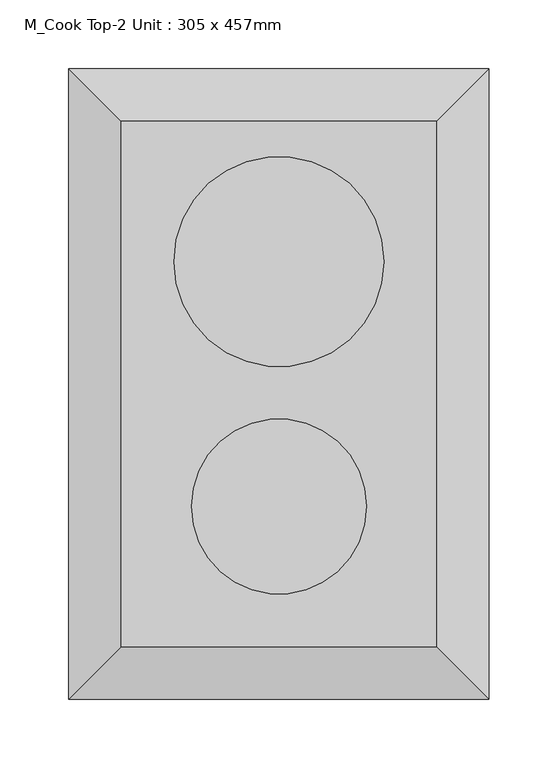
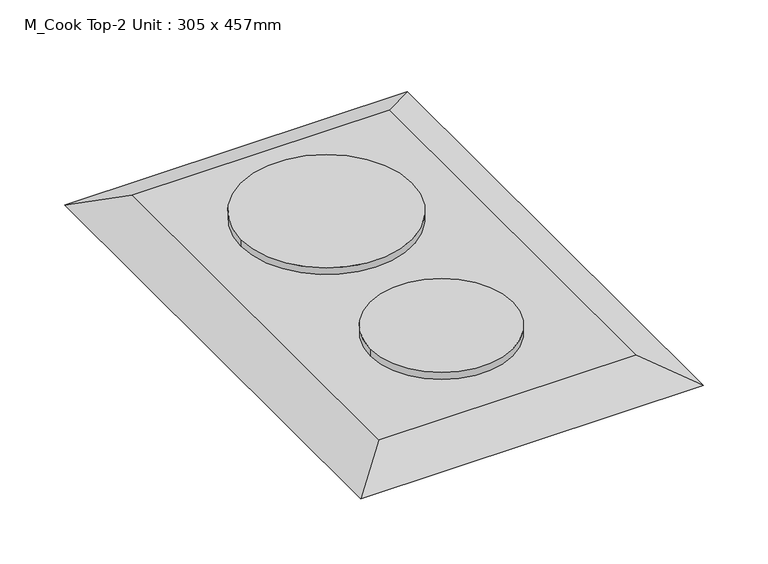
"""IFC4 building model written with IfcOpenShell, lengths in millimetres: proxy geometry, M_Cook Top-2 Unit : 305 x 457mm."""

from ifc_helpers import new_model, si_unit, point, frame, frame_2d, origin, place, context, project, spatial, circle_curve, trimmed, segment, composite_curve, outline, extrude, faceted_brep, source, transform, mapped, element, save


def m_cook_top_2_unit_305_x_457mm_ebea1746(model_context):
    return source(origin(), model_context, "Body", "SolidModel", [
        extrude(outline(composite_curve([segment(trimmed(circle_curve(frame_2d((76.2, 119.0247956)), 76.2), [point((152.4, 119.0247956))], [point((0.0, 119.0247956))], False, "CARTESIAN"), True, "CONTINUOUS"), segment(trimmed(circle_curve(frame_2d((76.2, 119.0247956)), 76.2), [point((0.0, 119.0247956))], [point((152.4, 119.0247956))], False, "CARTESIAN"), True, "CONTINUOUS")], self_intersect=False)), frame((0.0, 0.0, 919.05), z_axis=(0.0, 0.0, 1.0), x_axis=(1.0, 0.0, 0.0)), (0.0, 0.0, 1.0), 6.35),
        extrude(outline(composite_curve([segment(trimmed(circle_curve(frame_2d((76.2, -58.5752044)), 63.5), [point((139.7, -58.5752044))], [point((12.7, -58.5752044))], False, "CARTESIAN"), True, "CONTINUOUS"), segment(trimmed(circle_curve(frame_2d((76.2, -58.5752044)), 63.5), [point((12.7, -58.5752044))], [point((139.7, -58.5752044))], False, "CARTESIAN"), True, "CONTINUOUS")], self_intersect=False)), frame((0.0, 0.0, 919.05), z_axis=(0.0, 0.0, 1.0), x_axis=(1.0, 0.0, 0.0)), (0.0, 0.0, 1.0), 6.35),
        faceted_brep([(190.6, 220.6247956, 919.05), (-38.2, 220.6247956, 919.05), (-38.2, -160.1752044, 919.05), (190.6, -160.1752044, 919.05), (228.7, 258.7247956, 900.0), (228.7, -198.2752044, 900.0), (-76.3, -198.2752044, 900.0), (-76.3, 258.7247956, 900.0)], [[[0, 1, 2, 3]], [[4, 5, 6, 7]], [[4, 7, 1, 0]], [[7, 6, 2, 1]], [[6, 5, 3, 2]], [[5, 4, 0, 3]]]),
    ])


if __name__ == "__main__":
    model = new_model("IFC4")
    model_context = context("Model", 3, world=origin())
    ifc_project = project(units=[si_unit("LENGTHUNIT", "METRE", prefix="MILLI")], contexts=[model_context])
    site = spatial("IfcSite", under=ifc_project)
    building = spatial("IfcBuilding", under=site)
    placement = place(None, origin())
    m_cook_top_2_unit_305_x_457mm_shape = m_cook_top_2_unit_305_x_457mm_ebea1746(model_context)
    element("IfcBuildingElementProxy", 1, Name="M_Cook Top-2 Unit : 305 x 457mm", ObjectType="M_Cook Top-2 Unit : 305 x 457mm", at=placement, inside=building, context=model_context, shape_type="MappedRepresentation", body=[
        mapped(m_cook_top_2_unit_305_x_457mm_shape, transform((0.0, 0.0, 0.0), x_axis=(1.0, 0.0, 0.0), y_axis=(0.0, 1.0, 0.0), z_axis=(0.0, 0.0, 1.0))),
    ])
    save(model, "model.ifc")

# Revit data of these elements
# Type "M_Cook Top-2 Unit : 305 x 457mm"
#   Counter Height = 900 mm
#   Depth = 457 mm
#   Width = 305 mm
#   Burner Material = Steel, Chrome Plated
#   Cooktop Material = Steel, Polished
#   Default Elevation = 0
# Element 1 (IfcBuildingElementProxy, "M_Cook Top-2 Unit : 305 x 457mm")
#   Materials on its faces: "Steel, Chrome Plated", "Steel, Polished"
# Materials
#   "Steel, Chrome Plated": class "Metal", colour RGB 244 244 244, transparency 0, Description = "Chromiuim plated steel", Cost = 0
#   "Steel, Polished": class "Metal", colour RGB 57 57 57, transparency 0, Description = "Polished steel", Cost = 0
